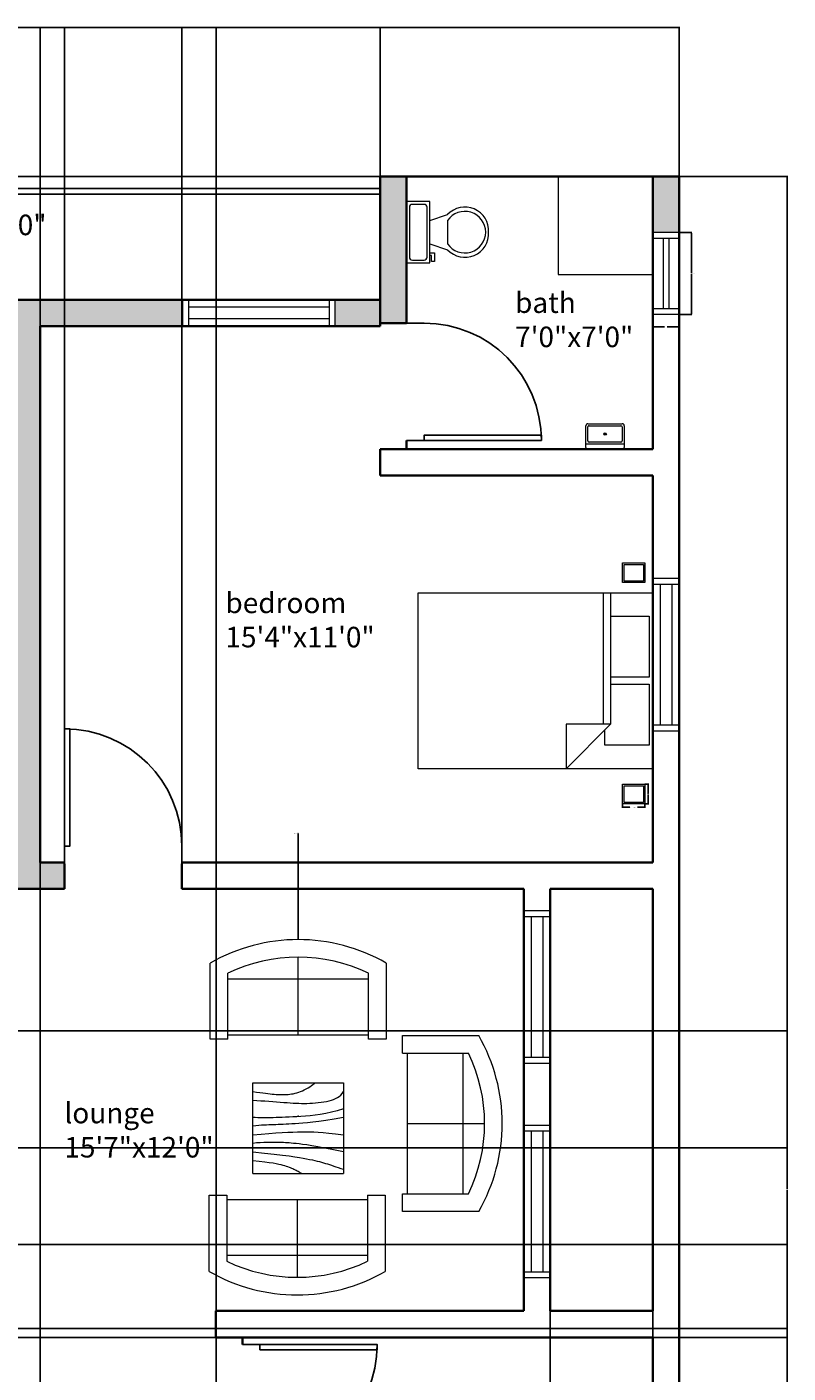
# Model space of a CAD drawing. Units: inches. Extents: x 1801 to 2333, y 478 to 1258.
# Tile 3 of 3: x 2074 to 2333, y 798 to 1258. Entities that reach past the tile are written whole.
import ezdxf

# ---------------------------------------------------------------- set-up
doc = ezdxf.new("R2010")
doc.units = ezdxf.units.IN
doc.header["$MEASUREMENT"] = 0
for name, color, linetype, lineweight in [('A-ANNO-DIMS', 2, 'Continuous', 18), ('A-AREA-IDEN', 7, 'Continuous', 18), ('A-DOOR', 4, 'Continuous', 25), ('A-FLOR-FIXT', 9, 'Continuous', 18), ('A-FURN', 8, 'Continuous', 18), ('A-GLAZ', 4, 'Continuous', 18), ('A-WALL', 7, 'Continuous', 35), ('A-WALL-PATT', 252, 'Continuous', 13), ('C-PROP', 3, 'Continuous', 25)]:
    doc.layers.add(name, color=color, linetype=linetype, lineweight=lineweight)
doc.styles.get("Standard").update_dxf_attribs({"font": 'arial.ttf'})
doc.dimstyles.get("Standard").update_dxf_attribs({"dimtxt": 0.18, "dimasz": 0.18, "dimexe": 0.18, "dimexo": 0.0625, "dimgap": 0.09, "dimtad": 0, "dimtih": 1, "dimtoh": 1, "dimdec": 0, "dimzin": 0, "dimdsep": 46, "dimlunit": 3, "dimtxsty": 'Standard', "dimcen": 0.09, "dimadec": 0, "dimazin": 0, "dimtfac": 1, "dimtdec": 0, "dimtofl": 0, "dimtmove": 0, "dimatfit": 3, "dimfxl": 1, "dimtolj": 1, "dimtzin": 0, "dimarcsym": 0})

# ---------------------------------------------------------------- blocks, each defined once
blk = doc.blocks.new('*U2')
for p, q in [((0, 0), (0, -6)), ((40, 0), (40, -6))]:
    blk.add_line(p, q)
blk.add_lwpolyline([(0, 0), (0, 40), (1.75, 40), (1.75, 0)], close=True)
blk.add_arc((0, 0), 40, 0, 90)
blk = doc.blocks.new('*U6')
for p, q in [((241.3, -152.4), (241.3, -50.8)), ((-254, -215.9), (-203.2, -215.9)), ((-254, -241.3), (-254, -215.9)), ((-203.2, -215.9), (-203.2, -203.2)), ((-177.8, -203.2), (-177.8, -241.3)), ((-101.6, -203.2), (-152.4, -355.6)), ((101.6, -203.2), (152.4, -355.6)), ((-177.8, -241.3), (-254, -241.3)), ((101.6, -355.6), (-101.6, -355.6))]:
    blk.add_line(p, q)
blk.add_lwpolyline([(266.7, -203.2), (266.7, 0), (-266.7, 0), (-266.7, -203.2)], close=True)
for points in [[(-241.3, -50.8), (-241.3, -152.4)], [(215.9, -25.4), (-215.9, -25.4)], [(-215.9, -177.8), (215.9, -177.8)]]:
    blk.add_lwpolyline(points)
for centre, radius, start, end in [((-219.075, -47.625), 22.45064, 81.8699, 188.1301), ((219.075, -47.625), 22.45064, 351.8699, 98.1301), ((-219.075, -155.575), 22.45064, 171.869898, 278.1301), ((219.075, -155.575), 22.45064, 261.8699, 8.1301), ((-12.12088, -505.93752), 205.61935, 133.01722, 273.38), ((0.94996, -504.77674), 181.02486, 124.50543, 269.7), ((-0.94742, -504.77674), 181.02486, 270.3, 55.4946), ((12.12342, -505.93752), 205.61935, 266.62, 46.9828)]:
    blk.add_arc(centre, radius, start, end)
blk = doc.blocks.new('Table - Square Woodgrain 42 x 42 in.')
blk.add_line((0, -42), (42, -42))
for points in [[(0, -4), (1.704, -4.2172), (3.2358, -4.4188), (4.615, -4.604), (5.8615, -4.7721), (6.9951, -4.9224), (8.0357, -5.0541), (9.0031, -5.1667), (9.9171, -5.2594), (10.7951, -5.3316), (11.6445, -5.3836), (12.4702, -5.4157), (13.277, -5.4283), (14.0698, -5.4217), (14.8535, -5.3964), (15.6331, -5.3526), (16.4133, -5.2908), (17.1986, -5.2103), (17.9913, -5.1062), (18.793, -4.9727), (19.6056, -4.8038), (20.4307, -4.5937), (21.2701, -4.3365), (22.1256, -4.0262), (22.9989, -3.6571), (23.888, -3.2272), (24.7756, -2.7516), (25.6408, -2.2491), (26.4624, -1.7387), (27.2195, -1.2395), (27.891, -0.7703), (28.456, -0.3501), (28.8934, 0.002)], [(0, -42), (0, 0), (42, 0), (42, -42)], [(0, -8), (1.8203, -8.1001), (3.6741, -8.2149), (5.5411, -8.3408), (7.4011, -8.4741), (9.2339, -8.6112), (11.0193, -8.7484), (12.7371, -8.8821), (14.3671, -9.0086), (15.8954, -9.1246), (17.3337, -9.2278), (18.6997, -9.3159), (20.0116, -9.387), (21.2871, -9.4389), (22.5442, -9.4696), (23.8008, -9.477), (25.0749, -9.459), (26.3791, -9.4137), (27.7049, -9.3403), (29.0383, -9.2382), (30.3655, -9.1068), (31.6728, -8.9455), (32.9461, -8.7535), (34.1717, -8.5304), (35.3358, -8.2756), (36.4268, -7.9863), (37.443, -7.6521), (38.3849, -7.2603), (39.253, -6.7986), (40.048, -6.2542), (40.7705, -5.6147), (41.421, -4.8674), (42, -4)], [(42, -12), (39.1784, -12.8621), (36.4519, -13.5654), (33.8246, -14.1294), (31.3004, -14.5731), (28.8832, -14.9161), (26.577, -15.1775), (24.3858, -15.3768), (22.3136, -15.5332), (20.3622, -15.6632), (18.5254, -15.7718), (16.7947, -15.8612), (15.1618, -15.9338), (13.6183, -15.9916), (12.1558, -16.0369), (10.7659, -16.0718), (9.4403, -16.0987), (8.1703, -16.1191), (6.9461, -16.1325), (5.7577, -16.1377), (4.595, -16.1335), (3.4479, -16.1188), (2.3064, -16.0924), (1.1604, -16.0532), (0, -16)], [(42, -16), (37.6529, -16.7365), (33.8802, -17.329), (30.6179, -17.7961), (27.8015, -18.1561), (25.3668, -18.4275), (23.2497, -18.6288), (21.3859, -18.7785), (19.7111, -18.8949), (18.1693, -18.9939), (16.7375, -19.0795), (15.401, -19.1534), (14.1449, -19.217), (12.9544, -19.2717), (11.8148, -19.3191), (10.7113, -19.3606), (9.6291, -19.3976), (8.5534, -19.4323), (7.47, -19.4689), (6.3643, -19.5122), (5.222, -19.5672), (4.0288, -19.6386), (2.7703, -19.7313), (1.4321, -19.8501), (0, -20)], [(0, -24), (3.9243, -23.6805), (7.4766, -23.4138), (10.6891, -23.1954), (13.5943, -23.0205), (16.2247, -22.8847), (18.6125, -22.7832), (20.7903, -22.7116), (22.7903, -22.6651), (24.6563, -22.642), (26.4764, -22.6507), (28.35, -22.7024), (30.3766, -22.8084), (32.6555, -22.98), (35.2861, -23.2283), (38.3678, -23.5645), (42, -24)], [(42, -32), (37.392, -31.017), (33.4585, -30.2231), (30.1291, -29.5949), (27.3334, -29.109), (25.0009, -28.742), (23.0612, -28.4707), (21.4439, -28.2716), (20.0786, -28.1215), (18.8998, -28.0002), (17.8609, -27.9014), (16.9206, -27.8219), (16.0371, -27.7588), (15.1691, -27.709), (14.2748, -27.6693), (13.3128, -27.6368), (12.2415, -27.6083), (11.0295, -27.5824), (9.6867, -27.5643), (8.233, -27.5608), (6.6884, -27.5787), (5.0728, -27.6248), (3.4062, -27.7058), (1.7086, -27.8286), (0, -28)], [(0, -32), (5.4026, -32.5358), (9.9494, -33.019), (13.7424, -33.4553), (16.8834, -33.8505), (19.4743, -34.2106), (21.6171, -34.5413), (23.4136, -34.8486), (24.9657, -35.1382), (26.3614, -35.4156), (27.6332, -35.6841), (28.7995, -35.9467), (29.8788, -36.2064), (30.8897, -36.4661), (31.8507, -36.7288), (32.7802, -36.9973), (33.6968, -37.2747), (34.6175, -37.5635), (35.5531, -37.8651), (36.5128, -38.1805), (37.506, -38.5108), (38.5421, -38.8568), (39.6302, -39.2197), (40.7797, -39.6004), (42, -40)], [(0, -36), (3.0098, -36.2857), (5.5354, -36.5643), (7.6368, -36.8359), (9.374, -37.1009), (10.807, -37.3597), (11.9957, -37.6126), (13.0002, -37.8599), (13.8804, -38.102), (14.6874, -38.3393), (15.4365, -38.5729), (16.1338, -38.8041), (16.7858, -39.0341), (17.3987, -39.264), (17.9787, -39.4952), (18.5322, -39.7288), (19.0655, -39.9662), (19.5832, -40.2081), (20.0842, -40.4544), (20.5657, -40.7046), (21.0249, -40.9581), (21.459, -41.2144), (21.8653, -41.4731), (22.2409, -41.7335), (22.5831, -41.9951)]]:
    blk.add_lwpolyline(points)
blk = doc.blocks.new('Sink-single - 30 in top')
blk.add_line((-15, -3.999996), (15, -3.999996))
for points in [[(-13.5, 0), (13.5, 0)], [(-15, -18.499996), (-15, -1.5)], [(-13.5, -17.499996), (-13.5, -6.499996)], [(-12.5, -5.499996), (12.5, -5.499996)], [(13.5, -6.499996), (13.5, -17.499996)], [(15, -1.5), (15, -18.499996)], [(13.5, -19.999996), (-13.5, -19.999996)], [(12.5, -18.499996), (-12.5, -18.499996)]]:
    blk.add_lwpolyline(points)
for radius in [1, 0.5]:
    blk.add_circle((0, -11.999996), radius)
for centre, radius, start, end in [((-13.5, -1.5), 1.5, 90, 180), ((-12.5, -6.499996), 1, 90, 180), ((12.5, -6.499996), 1, 0, 90), ((13.5, -1.5), 1.5, 0, 90), ((-13.5, -18.499996), 1.5, 180, 270), ((-12.5, -17.499996), 1, 180, 270), ((12.5, -17.499996), 1, 270, 0), ((13.5, -18.499996), 1.5, 270, 0)]:
    blk.add_arc(centre, radius, start, end)
blk = doc.blocks.new('Sofa - Roundback Loveseat 5 ft.')
for p, q in [((0, -32.44198), (0, -5.99998)), ((-24, -33.99998), (-24, -11.46958)), ((-23.9998, -13.38178), (23.99986, -13.38178)), ((24.00004, -33.99998), (24.00004, -11.46958)), ((-24, -32.44198), (24.00004, -32.44198))]:
    blk.add_line(p, q)
for points in [[(-24, -33.99998), (-30, -33.99998), (-30, -7.99998)], [(30.00004, -7.99998), (30.00004, -33.99998), (24.00004, -33.99998)]]:
    blk.add_lwpolyline(points)
for centre, radius, start, end in [((0, -60.24998), 60.24998, 60.13715, 119.8628), ((0, -61.38438), 55.38444, 64.32083, 115.6792)]:
    blk.add_arc(centre, radius, start, end)
blk = doc.blocks.new('Bed - Queen')
for p, q in [((0, -80.00003), (0, 0)), ((0, 0), (59.99999, 0)), ((59.99999, 0), (59.99999, -80.00003)), ((7.99999, -1.2), (28.79998, -1.2)), ((7.99999, -14.4), (7.99999, -1.2)), ((28.79998, -1.2), (28.79998, -14.4)), ((31.19999, -1.2), (51.99999, -1.2)), ((31.19999, -14.4), (31.19999, -1.2)), ((51.99999, -1.2), (51.99999, -16.4)), ((0, -14.4), (44.8, -14.4)), ((44.8, -16.8), (0, -16.8)), ((59.99999, -29.6), (44.8, -14.4)), ((44.8, -14.4), (44.8, -29.6)), ((51.99999, -16.4), (46.79936, -16.4)), ((44.8, -29.6), (59.99999, -29.6)), ((59.99999, -80.00003), (0, -80.00003))]:
    blk.add_line(p, q)
blk = doc.blocks.new('WIN-48IN')
for p, q in [((0, 0), (0, 9)), ((2, 0), (2, 9)), ((2, 6.5), (50, 6.5)), ((50, 0), (50, 9)), ((52, 0), (52, 9)), ((2, 2.5), (50, 2.5))]:
    blk.add_line(p, q)
blk = doc.blocks.new('WIN-24IN')
for p, q in [((9, 28), (0, 28)), ((9, 26), (0, 26)), ((3.5, 26), (3.5, 2)), ((5.5, 26), (5.5, 2)), ((9, 2), (0, 2)), ((9, 0), (0, 0))]:
    blk.add_line(p, q)
blk = doc.blocks.new('BEDSIDE-STAND')
for points in [[(0, 6.71), (7.61, 6.71), (7.61, 0), (0, 0)], [(0.62, 6.12), (7.2, 6.12), (7.2, 0.48), (0.62, 0.48)]]:
    blk.add_lwpolyline(points, close=True)
blk = doc.blocks.new('*D19')
at = {"layer": 'A-ANNO-DIMS', "color": 0, "lineweight": -2, "transparency": 16777216}
for p, q in [((2296.35, 1187.41), (2300.67, 1187.41)), ((2300.49, 1187.23), (2300.49, 1173.59)), ((2300.49, 1159.59), (2300.49, 1173.22)), ((2296.35, 1159.41), (2300.67, 1159.41))]:
    blk.add_line(p, q, dxfattribs=at)
at = {"layer": 'A-ANNO-DIMS', "color": 0, "transparency": 16777216}
for points in [[(2300.46, 1187.23), (2300.52, 1187.23), (2300.49, 1187.41)], [(2300.46, 1159.59), (2300.52, 1159.59), (2300.49, 1159.41)]]:
    blk.add_solid(points, dxfattribs=at)
at = {"layer": 'Defpoints', "color": 0, "transparency": 16777216}
for p in [(2296.29, 1187.41), (2300.49, 1187.41), (2296.29, 1159.41)]:
    blk.add_point(p, dxfattribs=at)
at = {"layer": 'A-ANNO-DIMS', "color": 0, "transparency": 16777216, "insert": (2300.49, 1173.41), "char_height": 0.18, "attachment_point": 5}
blk.add_mtext('\\A1;BATH WINDOW 28 TYP.', dxfattribs=at)
blk = doc.blocks.new('*D20')
at = {"layer": 'A-ANNO-DIMS', "color": 0, "lineweight": -2, "transparency": 16777216}
for p, q in [((2287.29, 1159.34), (2287.29, 1155.03)), ((2296.29, 1159.34), (2296.29, 1155.03)), ((2287.47, 1155.21), (2291.33, 1155.21)), ((2296.11, 1155.21), (2292.25, 1155.21))]:
    blk.add_line(p, q, dxfattribs=at)
at = {"layer": 'A-ANNO-DIMS', "color": 0, "transparency": 16777216}
for points in [[(2287.47, 1155.24), (2287.47, 1155.18), (2287.29, 1155.21)], [(2296.11, 1155.24), (2296.11, 1155.18), (2296.29, 1155.21)]]:
    blk.add_solid(points, dxfattribs=at)
at = {"layer": 'Defpoints', "color": 0, "transparency": 16777216}
for p in [(2287.29, 1159.41), (2296.29, 1159.41), (2296.29, 1155.21)]:
    blk.add_point(p, dxfattribs=at)
at = {"layer": 'A-ANNO-DIMS', "color": 0, "transparency": 16777216, "insert": (2291.79, 1155.21), "char_height": 0.18, "attachment_point": 5}
blk.add_mtext('\\A1;9 TYP.', dxfattribs=at)
blk = doc.blocks.new('*D25')
at = {"layer": 'A-ANNO-DIMS', "color": 0, "lineweight": -2, "transparency": 16777216}
for p, q in [((2276.96, 992.41), (2276.96, 991.15)), ((2284.57, 992.41), (2284.57, 991.15)), ((2277.14, 991.33), (2279.46, 991.33)), ((2284.39, 991.33), (2282.07, 991.33))]:
    blk.add_line(p, q, dxfattribs=at)
at = {"layer": 'A-ANNO-DIMS', "color": 0, "transparency": 16777216}
for points in [[(2277.14, 991.36), (2277.14, 991.3), (2276.96, 991.33)], [(2284.39, 991.36), (2284.39, 991.3), (2284.57, 991.33)]]:
    blk.add_solid(points, dxfattribs=at)
at = {"layer": 'Defpoints', "color": 0, "transparency": 16777216}
for p in [(2276.96, 992.47), (2284.57, 992.47), (2284.57, 991.33)]:
    blk.add_point(p, dxfattribs=at)
at = {"layer": 'A-ANNO-DIMS', "color": 0, "transparency": 16777216, "insert": (2280.76, 991.33), "char_height": 0.18, "attachment_point": 5}
blk.add_mtext('\\A1;NIGHTSTAND 8 TYP.', dxfattribs=at)
blk = doc.blocks.new('*D26')
at = {"layer": 'A-ANNO-DIMS', "color": 0, "lineweight": -2, "transparency": 16777216}
for p, q in [((2284.63, 999.18), (2285.89, 999.18)), ((2285.71, 999), (2285.71, 996.01)), ((2284.63, 992.47), (2285.89, 992.47)), ((2285.71, 992.65), (2285.71, 995.65))]:
    blk.add_line(p, q, dxfattribs=at)
at = {"layer": 'A-ANNO-DIMS', "color": 0, "transparency": 16777216}
for points in [[(2285.68, 999), (2285.74, 999), (2285.71, 999.18)], [(2285.68, 992.65), (2285.74, 992.65), (2285.71, 992.47)]]:
    blk.add_solid(points, dxfattribs=at)
at = {"layer": 'Defpoints', "color": 0, "transparency": 16777216}
for p in [(2284.57, 999.18), (2285.71, 999.18), (2284.57, 992.47)]:
    blk.add_point(p, dxfattribs=at)
at = {"layer": 'A-ANNO-DIMS', "color": 0, "transparency": 16777216, "insert": (2285.71, 995.83), "char_height": 0.18, "attachment_point": 5}
blk.add_mtext('\\A1;7 TYP.', dxfattribs=at)
blk = doc.blocks.new('*D35')
at = {"layer": 'A-ANNO-DIMS', "color": 0, "lineweight": -2, "transparency": 16777216}
for p, q in [((1838.29, 1202.54), (1838.29, 1257.55)), ((1838.47, 1257.37), (2067, 1257.37)), ((2296.11, 1257.37), (2067.58, 1257.37)), ((2296.29, 1206.54), (2296.29, 1257.55))]:
    blk.add_line(p, q, dxfattribs=at)
at = {"layer": 'A-ANNO-DIMS', "color": 0, "transparency": 16777216}
for points in [[(1838.47, 1257.4), (1838.47, 1257.34), (1838.29, 1257.37)], [(2296.11, 1257.4), (2296.11, 1257.34), (2296.29, 1257.37)]]:
    blk.add_solid(points, dxfattribs=at)
at = {"layer": 'Defpoints', "color": 0, "transparency": 16777216}
for p in [(2296.29, 1257.37), (2296.29, 1206.47), (1838.29, 1202.47)]:
    blk.add_point(p, dxfattribs=at)
at = {"layer": 'A-ANNO-DIMS', "color": 0, "transparency": 16777216, "insert": (2067.29, 1257.37), "char_height": 0.18, "attachment_point": 5}
blk.add_mtext('\\A1;458', dxfattribs=at)
blk = doc.blocks.new('*D36')
at = {"layer": 'A-ANNO-DIMS', "color": 0, "lineweight": -2, "transparency": 16777216}
for p, q in [((2296.35, 1206.47), (2333.32, 1206.47)), ((2333.14, 1206.29), (2333.14, 861.16)), ((2333.14, 515.65), (2333.14, 860.79)), ((2296.35, 515.47), (2333.32, 515.47))]:
    blk.add_line(p, q, dxfattribs=at)
at = {"layer": 'A-ANNO-DIMS', "color": 0, "transparency": 16777216}
for points in [[(2333.11, 1206.29), (2333.17, 1206.29), (2333.14, 1206.47)], [(2333.11, 515.65), (2333.17, 515.65), (2333.14, 515.47)]]:
    blk.add_solid(points, dxfattribs=at)
at = {"layer": 'Defpoints', "color": 0, "transparency": 16777216}
for p in [(2296.29, 1206.47), (2333.14, 1206.47), (2296.29, 515.47)]:
    blk.add_point(p, dxfattribs=at)
at = {"layer": 'A-ANNO-DIMS', "color": 0, "transparency": 16777216, "insert": (2333.14, 860.97), "char_height": 0.18, "attachment_point": 5}
blk.add_mtext('\\A1;691', dxfattribs=at)
blk = doc.blocks.new('*D40')
at = {"layer": 'A-ANNO-DIMS', "color": 0, "lineweight": -2, "transparency": 16777216}
for p, q in [((2069.29, 1155.54), (2069.29, 1257.55)), ((2069.47, 1257.37), (2131.51, 1257.37)), ((2194.11, 1257.37), (2132.07, 1257.37)), ((2194.29, 1164.54), (2194.29, 1257.55))]:
    blk.add_line(p, q, dxfattribs=at)
at = {"layer": 'A-ANNO-DIMS', "color": 0, "transparency": 16777216}
for points in [[(2069.47, 1257.4), (2069.47, 1257.34), (2069.29, 1257.37)], [(2194.11, 1257.4), (2194.11, 1257.34), (2194.29, 1257.37)]]:
    blk.add_solid(points, dxfattribs=at)
at = {"layer": 'Defpoints', "color": 0, "transparency": 16777216}
for p in [(2194.29, 1257.37), (2194.29, 1164.47), (2069.29, 1155.47)]:
    blk.add_point(p, dxfattribs=at)
at = {"layer": 'A-ANNO-DIMS', "color": 0, "transparency": 16777216, "insert": (2131.79, 1257.37), "char_height": 0.18, "attachment_point": 5}
blk.add_mtext('\\A1;125', dxfattribs=at)
blk = doc.blocks.new('*D41')
at = {"layer": 'A-ANNO-DIMS', "color": 0, "lineweight": -2, "transparency": 16777216}
for p, q in [((2287.35, 810.47), (2333.32, 810.47)), ((2333.14, 810.29), (2333.14, 692.16)), ((2333.14, 573.65), (2333.14, 691.79)), ((2287.35, 573.47), (2333.32, 573.47))]:
    blk.add_line(p, q, dxfattribs=at)
at = {"layer": 'A-ANNO-DIMS', "color": 0, "transparency": 16777216}
for points in [[(2333.11, 810.29), (2333.17, 810.29), (2333.14, 810.47)], [(2333.11, 573.65), (2333.17, 573.65), (2333.14, 573.47)]]:
    blk.add_solid(points, dxfattribs=at)
at = {"layer": 'Defpoints', "color": 0, "transparency": 16777216}
for p in [(2287.29, 810.47), (2333.14, 810.47), (2287.29, 573.47)]:
    blk.add_point(p, dxfattribs=at)
at = {"layer": 'A-ANNO-DIMS', "color": 0, "transparency": 16777216, "insert": (2333.14, 691.97), "char_height": 0.18, "attachment_point": 5}
blk.add_mtext('\\A1;237', dxfattribs=at)
blk = doc.blocks.new('*D44')
at = {"layer": 'A-ANNO-DIMS', "color": 0, "lineweight": -2, "transparency": 16777216}
for p, q in [((2194.23, 1206.47), (1801.26, 1206.47)), ((1801.44, 1206.29), (1801.44, 1185.66)), ((1801.44, 1164.65), (1801.44, 1185.29)), ((2194.23, 1164.47), (1801.26, 1164.47))]:
    blk.add_line(p, q, dxfattribs=at)
at = {"layer": 'A-ANNO-DIMS', "color": 0, "transparency": 16777216}
for points in [[(1801.41, 1206.29), (1801.47, 1206.29), (1801.44, 1206.47)], [(1801.41, 1164.65), (1801.47, 1164.65), (1801.44, 1164.47)]]:
    blk.add_solid(points, dxfattribs=at)
at = {"layer": 'Defpoints', "color": 0, "transparency": 16777216}
for p in [(1801.44, 1206.47), (2194.29, 1206.47), (2194.29, 1164.47)]:
    blk.add_point(p, dxfattribs=at)
at = {"layer": 'A-ANNO-DIMS', "color": 0, "transparency": 16777216, "insert": (1801.44, 1185.47), "char_height": 0.18, "attachment_point": 5}
blk.add_mtext('\\A1;42', dxfattribs=at)
blk = doc.blocks.new('*D46')
at = {"layer": 'A-ANNO-DIMS', "color": 0, "lineweight": -2, "transparency": 16777216}
for p, q in [((2252.29, 963.41), (2252.29, 478.11)), ((2287.29, 963.41), (2287.29, 478.11)), ((2252.47, 478.29), (2269.57, 478.29)), ((2287.11, 478.29), (2270.01, 478.29))]:
    blk.add_line(p, q, dxfattribs=at)
at = {"layer": 'A-ANNO-DIMS', "color": 0, "transparency": 16777216}
for points in [[(2252.47, 478.32), (2252.47, 478.26), (2252.29, 478.29)], [(2287.11, 478.32), (2287.11, 478.26), (2287.29, 478.29)]]:
    blk.add_solid(points, dxfattribs=at)
at = {"layer": 'Defpoints', "color": 0, "transparency": 16777216}
for p in [(2252.29, 963.47), (2287.29, 963.47), (2287.29, 478.29)]:
    blk.add_point(p, dxfattribs=at)
at = {"layer": 'A-ANNO-DIMS', "color": 0, "transparency": 16777216, "insert": (2269.79, 478.29), "char_height": 0.18, "attachment_point": 5}
blk.add_mtext('\\A1;35', dxfattribs=at)
blk = doc.blocks.new('*D47')
at = {"layer": 'A-ANNO-DIMS', "color": 0, "lineweight": -2, "transparency": 16777216}
for p, q in [((2086.64, 972.54), (2086.64, 1257.55)), ((2086.82, 1257.37), (2106.42, 1257.37)), ((2126.46, 1257.37), (2106.86, 1257.37)), ((2126.64, 972.54), (2126.64, 1257.55))]:
    blk.add_line(p, q, dxfattribs=at)
at = {"layer": 'A-ANNO-DIMS', "color": 0, "transparency": 16777216}
for points in [[(2086.82, 1257.4), (2086.82, 1257.34), (2086.64, 1257.37)], [(2126.46, 1257.4), (2126.46, 1257.34), (2126.64, 1257.37)]]:
    blk.add_solid(points, dxfattribs=at)
at = {"layer": 'Defpoints', "color": 0, "transparency": 16777216}
for p in [(2126.64, 1257.37), (2086.64, 972.47), (2126.64, 972.47)]:
    blk.add_point(p, dxfattribs=at)
at = {"layer": 'A-ANNO-DIMS', "color": 0, "transparency": 16777216, "insert": (2106.64, 1257.37), "char_height": 0.18, "attachment_point": 5}
blk.add_mtext('\\A1;40', dxfattribs=at)
blk = doc.blocks.new('*D48')
at = {"layer": 'A-ANNO-DIMS', "color": 0, "lineweight": -2, "transparency": 16777216}
for p, q in [((2147.23, 810.47), (1801.26, 810.47)), ((1801.44, 810.29), (1801.44, 789.42)), ((1801.44, 768.17), (1801.44, 789.05)), ((2147.23, 767.99), (1801.26, 767.99))]:
    blk.add_line(p, q, dxfattribs=at)
at = {"layer": 'A-ANNO-DIMS', "color": 0, "transparency": 16777216}
for points in [[(1801.41, 810.29), (1801.47, 810.29), (1801.44, 810.47)], [(1801.41, 768.17), (1801.47, 768.17), (1801.44, 767.99)]]:
    blk.add_solid(points, dxfattribs=at)
at = {"layer": 'Defpoints', "color": 0, "transparency": 16777216}
for p in [(1801.44, 810.47), (2147.29, 810.47), (2147.29, 767.99)]:
    blk.add_point(p, dxfattribs=at)
at = {"layer": 'A-ANNO-DIMS', "color": 0, "transparency": 16777216, "insert": (1801.44, 789.23), "char_height": 0.18, "attachment_point": 5}
blk.add_mtext('\\A1;42.48', dxfattribs=at)
blk = doc.blocks.new('*D51')
at = {"layer": 'A-ANNO-DIMS', "color": 0, "lineweight": -2, "transparency": 16777216}
for p, q in [((1982.97, 842.2), (2333.32, 842.2)), ((2333.14, 842.02), (2333.14, 828.02)), ((2333.14, 813.65), (2333.14, 827.65)), ((2005.35, 813.47), (2333.32, 813.47))]:
    blk.add_line(p, q, dxfattribs=at)
at = {"layer": 'A-ANNO-DIMS', "color": 0, "transparency": 16777216}
for points in [[(2333.11, 842.02), (2333.17, 842.02), (2333.14, 842.2)], [(2333.11, 813.65), (2333.17, 813.65), (2333.14, 813.47)]]:
    blk.add_solid(points, dxfattribs=at)
at = {"layer": 'Defpoints', "color": 0, "transparency": 16777216}
for p in [(1982.91, 842.2), (2005.29, 813.47), (2333.14, 813.47)]:
    blk.add_point(p, dxfattribs=at)
at = {"layer": 'A-ANNO-DIMS', "color": 0, "transparency": 16777216, "insert": (2333.14, 827.84), "char_height": 0.18, "attachment_point": 5}
blk.add_mtext('\\A1;28.72', dxfattribs=at)
blk = doc.blocks.new('*D54')
at = {"layer": 'A-ANNO-DIMS', "color": 0, "lineweight": -2, "transparency": 16777216}
for p, q in [((2005.35, 915.1), (2333.32, 915.1)), ((2333.14, 914.92), (2333.14, 895.29)), ((2333.14, 875.28), (2333.14, 894.92)), ((2005.35, 875.1), (2333.32, 875.1))]:
    blk.add_line(p, q, dxfattribs=at)
at = {"layer": 'A-ANNO-DIMS', "color": 0, "transparency": 16777216}
for points in [[(2333.11, 914.92), (2333.17, 914.92), (2333.14, 915.1)], [(2333.11, 875.28), (2333.17, 875.28), (2333.14, 875.1)]]:
    blk.add_solid(points, dxfattribs=at)
at = {"layer": 'Defpoints', "color": 0, "transparency": 16777216}
for p in [(2005.29, 915.1), (2333.14, 915.1), (2005.29, 875.1)]:
    blk.add_point(p, dxfattribs=at)
at = {"layer": 'A-ANNO-DIMS', "color": 0, "transparency": 16777216, "insert": (2333.14, 895.1), "char_height": 0.18, "attachment_point": 5}
blk.add_mtext('\\A1;40', dxfattribs=at)
blk = doc.blocks.new('*D59')
at = {"layer": 'A-ANNO-DIMS', "color": 0, "lineweight": -2, "transparency": 16777216}
for p, q in [((2078.29, 762.54), (2078.29, 1257.55)), ((2078.47, 1257.37), (2108.07, 1257.37)), ((2138.11, 1257.37), (2108.51, 1257.37)), ((2138.29, 762.54), (2138.29, 1257.55))]:
    blk.add_line(p, q, dxfattribs=at)
at = {"layer": 'A-ANNO-DIMS', "color": 0, "transparency": 16777216}
for points in [[(2078.47, 1257.4), (2078.47, 1257.34), (2078.29, 1257.37)], [(2138.11, 1257.4), (2138.11, 1257.34), (2138.29, 1257.37)]]:
    blk.add_solid(points, dxfattribs=at)
at = {"layer": 'Defpoints', "color": 0, "transparency": 16777216}
for p in [(2138.29, 1257.37), (2078.29, 762.47), (2138.29, 762.47)]:
    blk.add_point(p, dxfattribs=at)
at = {"layer": 'A-ANNO-DIMS', "color": 0, "transparency": 16777216, "insert": (2108.29, 1257.37), "char_height": 0.18, "attachment_point": 5}
blk.add_mtext('\\A1;60', dxfattribs=at)
blk = doc.blocks.new('*D61')
at = {"layer": 'A-ANNO-DIMS', "color": 0, "lineweight": -2, "transparency": 16777216}
for p, q in [((2166.17, 982.32), (2166.35, 982.32)), ((2166.35, 982.32), (2166.35, 946.35)), ((2166.26, 885.92), (2166.44, 885.92)), ((2166.35, 885.83), (2166.35, 886.01))]:
    blk.add_line(p, q, dxfattribs=at)
at = {"layer": 'A-ANNO-DIMS', "color": 0, "transparency": 16777216}
blk.add_solid([(2166.38, 946.35), (2166.32, 946.35), (2166.35, 946.17)], dxfattribs=at)
at = {"layer": 'Defpoints', "color": 0, "transparency": 16777216}
for p in [(2166.35, 946.17), (2166.35, 885.92)]:
    blk.add_point(p, dxfattribs=at)
at = {"layer": 'A-ANNO-DIMS', "color": 0, "transparency": 16777216, "insert": (2165.49, 982.32), "char_height": 0.18, "attachment_point": 5}
blk.add_mtext('\\A1;5X R60.25', dxfattribs=at)

msp = doc.modelspace()

# ---------------------------------------------------------------- hatches: boundary and pattern name
at = {"layer": 'A-WALL-PATT'}
h = msp.add_hatch(color=256, dxfattribs=at)
h.dxf.hatch_style = 1
h.paths.add_polyline_path([(1951.2881, 1164.4747), (1876.2881, 1164.4747), (1876.2881, 1110.5123), (1885.2881, 1110.5123), (1885.2881, 1155.4747), (1951.2881, 1155.4747)])
h.paths.add_polyline_path([(2126.8707, 1164.4747), (2003.2881, 1164.4747), (2003.2881, 1155.4747), (2069.2881, 1155.4747), (2069.2881, 1011.4747), (2064.4791, 1011.4747), (2064.4791, 1002.4747), (2069.2881, 1002.4747), (2069.2881, 963.4747), (2078.3234, 963.4747), (2086.6392, 963.4747), (2086.6392, 972.4747), (2078.3234, 972.4747), (2078.2881, 1002.4747), (2078.2881, 1155.4747), (2126.8707, 1155.4747)])
h.paths.add_polyline_path([(2194.2881, 1164.4747), (2178.8707, 1164.4747), (2178.8707, 1155.4747), (2194.2881, 1155.4747)])
h.paths.add_polyline_path([(2203.2881, 1206.4747), (2194.2881, 1206.4747), (2194.2881, 1156.4812), (2203.2881, 1156.4812)])
h.paths.add_polyline_path([(2296.2881, 1206.4747), (2287.2881, 1206.4747), (2287.2881, 1187.4062), (2296.2881, 1187.4062)])

# ---------------------------------------------------------------- linework, layer by layer
at = {"layer": 'A-FLOR-FIXT'}
msp.add_lwpolyline([(2287.2881, 1206.4747), (2254.9723, 1206.4747), (2254.9723, 1173.0681), (2287.2881, 1173.0681)], close=True, dxfattribs=at)
at = {"layer": 'A-GLAZ'}
for p, q in [((2287.2881, 1069.4471), (2296.2881, 1069.4471)), ((2287.2881, 1017.4471), (2296.2881, 1017.4471))]:
    msp.add_line(p, q, dxfattribs=at)
at = {"layer": 'A-WALL'}
for p, q in [((2194.2881, 1206.4747), (2296.2881, 1206.4747)), ((2194.2881, 1206.4747), (2194.2881, 1155.4747)), ((2194.2881, 1206.4747), (2194.2881, 1155.4747)), ((2203.2881, 1206.4747), (2203.2881, 1156.4812)), ((2287.2881, 1206.4747), (2287.2881, 1113.4747)), ((2296.2881, 1206.4747), (2296.2881, 517.4747)), ((1876.2881, 1164.4747), (2194.2881, 1164.4747)), ((2078.2881, 1002.4747), (2078.2881, 1155.4747)), ((2078.2881, 1155.4747), (2194.2881, 1155.4747)), ((2203.2881, 1156.4812), (2194.2881, 1156.4812)), ((2203.2881, 1116.4812), (2203.2881, 1113.4747)), ((2194.2881, 1113.4747), (2287.2881, 1113.4747)), ((2194.2881, 1113.4747), (2194.2881, 1104.4747)), ((2194.2881, 1104.4747), (2287.2881, 1104.4747)), ((2287.2881, 1104.4747), (2287.2881, 972.4747)), ((2078.2881, 1002.4747), (2078.3234, 972.4747)), ((2086.6392, 972.4747), (2078.3234, 972.4747)), ((2086.6392, 972.0449), (2086.6392, 963.4747)), ((2203.2881, 972.4747), (2126.6392, 972.4747)), ((2126.6392, 972.0449), (2126.6392, 963.4747)), ((2203.2881, 972.4747), (2287.2881, 972.4747)), ((2069.2881, 963.4747), (2078.3234, 963.4747)), ((2086.6392, 963.4747), (2078.3234, 963.4747)), ((2203.2881, 963.4747), (2126.6392, 963.4747)), ((2203.2881, 963.4747), (2243.2853, 963.4747)), ((2243.2853, 963.4747), (2243.2853, 819.4747)), ((2252.2853, 963.4747), (2252.2853, 819.4747)), ((2252.2853, 963.4747), (2287.2881, 963.4747)), ((2287.2881, 963.4747), (2287.2881, 819.4747)), ((2243.2853, 819.4747), (2138.2881, 819.4747)), ((2138.2881, 819.4747), (2138.2881, 810.4747)), ((2287.2881, 819.4747), (2252.2853, 819.4747)), ((2287.2881, 810.4747), (2138.2881, 810.4747)), ((2147.2881, 807.9929), (2147.2881, 810.4747)), ((2287.2881, 810.4747), (2287.2881, 573.4747))]:
    msp.add_line(p, q, dxfattribs=at)
at = {"layer": 'C-PROP'}
for p, q in [((1838.2881, 1202.4747), (2194.2881, 1202.4747)), ((1840.2881, 1200.4747), (2194.2881, 1200.4747))]:
    msp.add_line(p, q, dxfattribs=at)

# ---------------------------------------------------------------- block references
at = {"layer": 'A-DOOR', "xscale": -1, "rotation": 270}
msp.add_blockref('*U2', (2209.2881, 1116.4812), dxfattribs=at)
at = {"layer": 'A-DOOR'}
msp.add_blockref('*U2', (2086.6392, 978.0449), dxfattribs=at)
at = {"layer": 'A-DOOR', "rotation": 270}
msp.add_blockref('*U2', (2153.2881, 807.9929), dxfattribs=at)
at = {"layer": 'A-FLOR-FIXT'}
for name, p, xscale, yscale, zscale, rotation in [('*U6', (2203.2881, 1187.5202), 0.0393700787401575, 0.0393700787401575, 0.0393700787401575, 90), ('Sink-single - 30 in top', (2271.0142, 1113.4665), 0.4346134936801766, 0.4346134936801766, 0.4346134936801766, 180)]:
    msp.add_blockref(name, p, dxfattribs=dict(at, xscale=xscale, yscale=yscale, zscale=zscale, rotation=rotation))
at = {"layer": 'A-FURN'}
for name, p in [('BEDSIDE-STAND', (2276.9174, 1067.9856)), ('BEDSIDE-STAND', (2276.9573, 992.471)), ('Sofa - Roundback Loveseat 5 ft.', (2166.3484, 946.1725))]:
    msp.add_blockref(name, p, dxfattribs=at)
for name, p, rotation in [('Bed - Queen', (2287.2881, 1064.469), 270), ('Sofa - Roundback Loveseat 5 ft.', (2235.9154, 883.4083), 270), ('Sofa - Roundback Loveseat 5 ft.', (2165.9959, 824.9594), 180)]:
    msp.add_blockref(name, p, dxfattribs=dict(at, rotation=rotation))
at = {"layer": 'A-FURN', "xscale": 0.7359782021052613, "yscale": 0.7359782021052613, "zscale": 0.7359782021052613}
msp.add_blockref('Table - Square Woodgrain 42 x 42 in.', (2150.838, 897.2648), dxfattribs=at)
at = {"layer": 'A-GLAZ'}
msp.add_blockref('WIN-24IN', (2287.2879, 1159.4064), dxfattribs=at)
for p, rotation in [((2178.8707, 1164.4745), 180), ((2287.2883, 1069.4472), 270.0000000000021), ((2243.2856, 956.0461), 270.000000000001), ((2243.2856, 882.8763), 270.0000000000011)]:
    msp.add_blockref('WIN-48IN', p, dxfattribs=dict(at, rotation=rotation))

# ---------------------------------------------------------------- texts
at = {"layer": 'A-AREA-IDEN', "char_height": 7, "attachment_point": 1}
for s, width, insert in [('back lawn 3\'0" wide', 84.800625, (2015.4244, 1193.499)), ('bath\\P7\'0"x7\'0"\\P  ', 106.765691, (2240.33, 1166.9648)), ('bedroom\\P15\'4"x11\'0"\\P  ', 106.765691, (2141.5106, 1064.55)), ('lounge\\P15\'7"x12\'0"\\P  ', 106.765691, (2086.5661, 890.4976))]:
    msp.add_mtext_dynamic_manual_height_columns(s, width=width, gutter_width=1, heights=[0], dxfattribs=dict(at, insert=insert))

# ---------------------------------------------------------------- dimensions: what is measured, and where the dimension line sits
at = {"layer": 'A-ANNO-DIMS'}
for base, p1, p2, picture, middle in [((2296.2881, 1257.3702), (1838.2881, 1202.4747), (2296.2881, 1206.4747), '*D35', (2067.2881, 1257.3702)), ((2194.2881, 1257.3702), (2069.2881, 1155.4747), (2194.2881, 1164.4747), '*D40', (2131.7881, 1257.3702)), ((2138.2881, 1257.3702), (2078.2881, 762.4747), (2138.2881, 762.4747), '*D59', (2108.2881, 1257.3702)), ((2126.6392, 1257.3702), (2086.6392, 972.4747), (2126.6392, 972.4747), '*D47', (2106.6392, 1257.3702)), ((2287.2881, 478.2946), (2252.2853, 963.4747), (2287.2881, 963.4747), '*D46', (2269.7867, 478.2946))]:
    dim = msp.add_linear_dim(base=base, p1=p1, p2=p2, dimstyle='Standard', override={"dimdec": 0, "dimlfac": 1, "dimrnd": 0, "dimzin": 0, "dimdsep": 46, "dimlunit": 2}, dxfattribs=at)
    dim.commit()
    dim.dimension.update_dxf_attribs({"geometry": picture, "text_midpoint": middle})
for base, p1, p2, override, picture, middle in [((1801.4381, 1206.4747), (2194.2881, 1164.4747), (2194.2881, 1206.4747), {"dimdec": 0, "dimlfac": 1, "dimrnd": 0, "dimzin": 0, "dimdsep": 46, "dimlunit": 2}, '*D44', (1801.4381, 1185.4747)), ((2333.1381, 1206.4747), (2296.2881, 515.4747), (2296.2881, 1206.4747), {"dimdec": 0, "dimlfac": 1, "dimrnd": 0, "dimzin": 0, "dimdsep": 46, "dimlunit": 2}, '*D36', (2333.1381, 860.9747)), ((2333.1381, 915.105), (2005.2881, 875.105), (2005.2881, 915.105), {"dimdec": 0, "dimlfac": 1, "dimrnd": 0, "dimzin": 0, "dimdsep": 46, "dimlunit": 2}, '*D54', (2333.1381, 895.105)), ((2333.1381, 813.4747), (1982.9092, 842.1967), (2005.2881, 813.4747), {"dimdec": 2, "dimlfac": 1, "dimrnd": 0, "dimzin": 0, "dimdsep": 46, "dimlunit": 2}, '*D51', (2333.1381, 827.8357)), ((1801.4381, 810.4747), (2147.2881, 767.9929), (2147.2881, 810.4747), {"dimdec": 2, "dimlfac": 1, "dimrnd": 0, "dimzin": 0, "dimdsep": 46, "dimlunit": 2}, '*D48', (1801.4381, 789.2338)), ((2333.1381, 810.4747), (2287.2881, 573.4747), (2287.2881, 810.4747), {"dimdec": 0, "dimlfac": 1, "dimrnd": 0, "dimzin": 0, "dimdsep": 46, "dimlunit": 2}, '*D41', (2333.1381, 691.9747))]:
    dim = msp.add_linear_dim(base=base, p1=p1, p2=p2, angle=90, dimstyle='Standard', override=override, dxfattribs=at)
    dim.commit()
    dim.dimension.update_dxf_attribs({"geometry": picture, "text_midpoint": middle})
for base, p1, p2, text, picture, middle in [((2300.4881, 1187.4062), (2296.2881, 1159.4062), (2296.2881, 1187.4062), 'BATH WINDOW <> TYP.', '*D19', (2300.4881, 1173.4062)), ((2285.708, 999.1805), (2284.5667, 992.4715), (2284.5667, 999.1805), '<> TYP.', '*D26', (2285.708, 995.826))]:
    dim = msp.add_linear_dim(base=base, p1=p1, p2=p2, angle=90, text=text, dimstyle='Standard', override={"dimdec": 0, "dimlfac": 1, "dimrnd": 0, "dimzin": 0, "dimdsep": 46, "dimlunit": 2}, dxfattribs=at)
    dim.commit()
    dim.dimension.update_dxf_attribs({"geometry": picture, "text_midpoint": middle})
for base, p1, p2, text, picture, middle in [((2296.2881, 1155.2062), (2287.2881, 1159.4062), (2296.2881, 1159.4062), '<> TYP.', '*D20', (2291.7881, 1155.2062)), ((2284.5667, 991.3301), (2276.9576, 992.4715), (2284.5667, 992.4715), 'NIGHTSTAND <> TYP.', '*D25', (2280.7622, 991.3301))]:
    dim = msp.add_linear_dim(base=base, p1=p1, p2=p2, text=text, dimstyle='Standard', override={"dimdec": 0, "dimlfac": 1, "dimrnd": 0, "dimzin": 0, "dimdsep": 46, "dimlunit": 2}, dxfattribs=at)
    dim.commit()
    dim.dimension.update_dxf_attribs({"geometry": picture, "text_midpoint": middle})
dim = msp.add_radius_dim(center=(2166.3484, 885.9225), mpoint=(2166.348, 946.1725), text='5X <>', dimstyle='Standard', override={"dimdec": 2, "dimlfac": 1, "dimrnd": 0, "dimzin": 0, "dimdsep": 46, "dimlunit": 2}, dxfattribs=at)
dim.commit()
dim.dimension.update_dxf_attribs({"geometry": '*D61', "text_midpoint": (2165.4939, 982.3225), "dimtype": 164})

doc.saveas('drawing.dxf')
